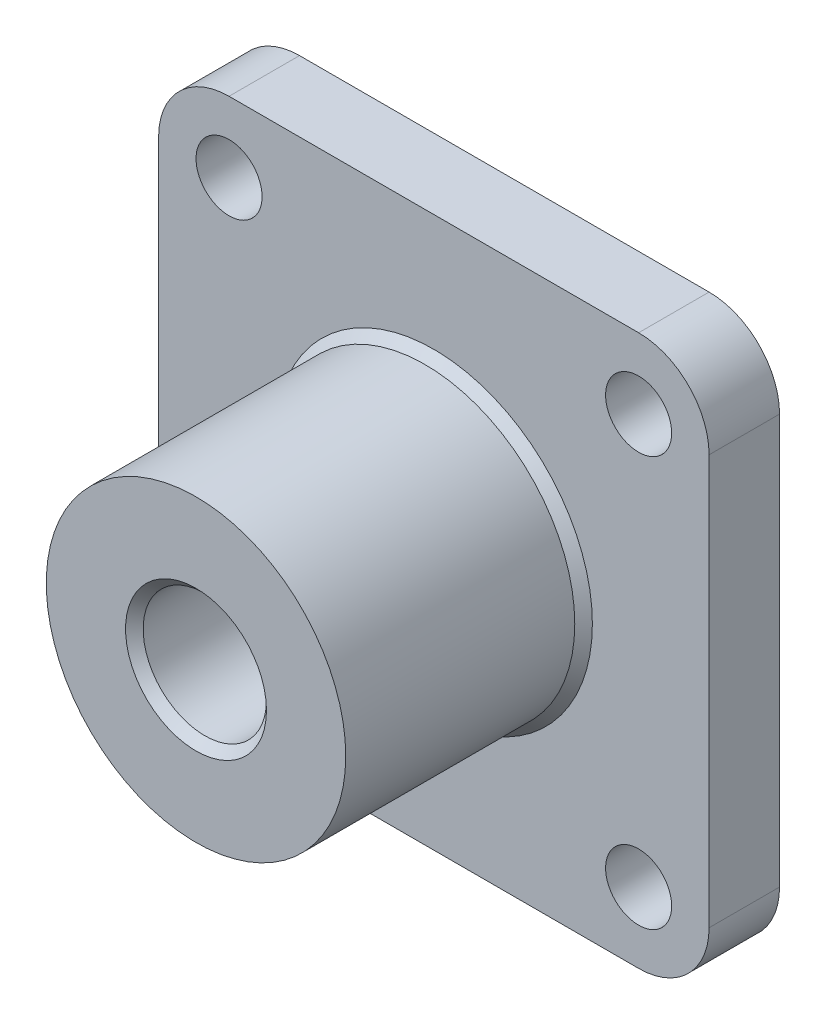
ISO-10303-21;
HEADER;
FILE_DESCRIPTION(('STEP AP214'),'2;1');
FILE_NAME('part.step','',(''),(''),'','','');
FILE_SCHEMA(('AUTOMOTIVE_DESIGN { 1 0 10303 214 1 1 1 1 }'));
ENDSEC;
DATA;
#1=APPLICATION_CONTEXT('core data for automotive mechanical design processes');
#2=APPLICATION_PROTOCOL_DEFINITION('international standard','automotive_design',2000,#1);
#3=PRODUCT_CONTEXT('',#1,'mechanical');
#4=PRODUCT('Part','Part','',(#3));
#5=PRODUCT_RELATED_PRODUCT_CATEGORY('part','',(#4));
#6=PRODUCT_DEFINITION_FORMATION('','',#4);
#7=PRODUCT_DEFINITION_CONTEXT('part definition',#1,'design');
#8=PRODUCT_DEFINITION('design','',#6,#7);
#9=PRODUCT_DEFINITION_SHAPE('','',#8);
#10=(LENGTH_UNIT() NAMED_UNIT(*) SI_UNIT(.MILLI.,.METRE.));
#11=(NAMED_UNIT(*) PLANE_ANGLE_UNIT() SI_UNIT($,.RADIAN.));
#12=(NAMED_UNIT(*) SI_UNIT($,.STERADIAN.) SOLID_ANGLE_UNIT());
#13=UNCERTAINTY_MEASURE_WITH_UNIT(LENGTH_MEASURE(1.E-05),#10,'distance_accuracy_value','');
#14=(GEOMETRIC_REPRESENTATION_CONTEXT(3) GLOBAL_UNCERTAINTY_ASSIGNED_CONTEXT((#13)) GLOBAL_UNIT_ASSIGNED_CONTEXT((#10,
#11,#12)) REPRESENTATION_CONTEXT('',''));
#15=CARTESIAN_POINT('',(0.,0.,0.));
#16=DIRECTION('',(0.,0.,1.));
#17=DIRECTION('',(1.,0.,0.));
#18=AXIS2_PLACEMENT_3D('',#15,#16,#17);
#19=CARTESIAN_POINT('',(16.,-109.,16.));
#20=DIRECTION('',(0.,0.,-1.));
#21=DIRECTION('',(-1.,0.,0.));
#22=AXIS2_PLACEMENT_3D('',#19,#20,#21);
#23=CYLINDRICAL_SURFACE('',#22,16.);
#24=CARTESIAN_POINT('',(16.,-109.,0.));
#25=DIRECTION('',(0.,0.,1.));
#26=DIRECTION('',(1.,0.,0.));
#27=AXIS2_PLACEMENT_3D('',#24,#25,#26);
#28=CIRCLE('',#27,16.);
#29=CARTESIAN_POINT('',(0.,-109.,0.));
#30=VERTEX_POINT('',#29);
#31=CARTESIAN_POINT('',(16.0000000000001,-125.,0.));
#32=VERTEX_POINT('',#31);
#33=EDGE_CURVE('E148',#30,#32,#28,.T.);
#34=ORIENTED_EDGE('',*,*,#33,.T.);
#35=DIRECTION('',(0.,0.,-1.));
#36=VECTOR('',#35,1.);
#37=CARTESIAN_POINT('',(16.0000000000001,-125.,16.));
#38=LINE('',#37,#36);
#39=CARTESIAN_POINT('',(16.0000000000001,-125.,16.));
#40=VERTEX_POINT('',#39);
#41=EDGE_CURVE('E174',#40,#32,#38,.T.);
#42=ORIENTED_EDGE('',*,*,#41,.F.);
#43=CARTESIAN_POINT('',(16.,-109.,16.));
#44=DIRECTION('',(0.,0.,1.));
#45=DIRECTION('',(1.,0.,0.));
#46=AXIS2_PLACEMENT_3D('',#43,#44,#45);
#47=CIRCLE('',#46,16.);
#48=CARTESIAN_POINT('',(0.,-109.,16.));
#49=VERTEX_POINT('',#48);
#50=EDGE_CURVE('E161',#49,#40,#47,.T.);
#51=ORIENTED_EDGE('',*,*,#50,.F.);
#52=DIRECTION('',(0.,0.,-1.));
#53=VECTOR('',#52,1.);
#54=CARTESIAN_POINT('',(0.,-109.,16.));
#55=LINE('',#54,#53);
#56=EDGE_CURVE('E142',#49,#30,#55,.T.);
#57=ORIENTED_EDGE('',*,*,#56,.T.);
#58=EDGE_LOOP('',(#34,#42,#51,#57));
#59=FACE_BOUND('',#58,.T.);
#60=ADVANCED_FACE('F50',(#59),#23,.T.);
#61=CARTESIAN_POINT('',(109.,-125.,16.));
#62=DIRECTION('',(0.,1.,0.));
#63=DIRECTION('',(0.,0.,1.));
#64=AXIS2_PLACEMENT_3D('',#61,#62,#63);
#65=PLANE('',#64);
#66=DIRECTION('',(1.,0.,0.));
#67=VECTOR('',#66,1.);
#68=CARTESIAN_POINT('',(109.,-125.,0.));
#69=LINE('',#68,#67);
#70=CARTESIAN_POINT('',(109.,-125.,0.));
#71=VERTEX_POINT('',#70);
#72=EDGE_CURVE('E149',#32,#71,#69,.T.);
#73=ORIENTED_EDGE('',*,*,#72,.T.);
#74=DIRECTION('',(0.,0.,-1.));
#75=VECTOR('',#74,1.);
#76=CARTESIAN_POINT('',(109.,-125.,16.));
#77=LINE('',#76,#75);
#78=CARTESIAN_POINT('',(109.,-125.,16.));
#79=VERTEX_POINT('',#78);
#80=EDGE_CURVE('E172',#79,#71,#77,.T.);
#81=ORIENTED_EDGE('',*,*,#80,.F.);
#82=DIRECTION('',(1.,0.,0.));
#83=VECTOR('',#82,1.);
#84=CARTESIAN_POINT('',(109.,-125.,16.));
#85=LINE('',#84,#83);
#86=EDGE_CURVE('E108',#40,#79,#85,.T.);
#87=ORIENTED_EDGE('',*,*,#86,.F.);
#88=ORIENTED_EDGE('',*,*,#41,.T.);
#89=EDGE_LOOP('',(#73,#81,#87,#88));
#90=FACE_BOUND('',#89,.T.);
#91=ADVANCED_FACE('F197',(#90),#65,.F.);
#92=CARTESIAN_POINT('',(109.,-109.,16.));
#93=DIRECTION('',(0.,0.,-1.));
#94=DIRECTION('',(-1.,0.,0.));
#95=AXIS2_PLACEMENT_3D('',#92,#93,#94);
#96=CYLINDRICAL_SURFACE('',#95,16.);
#97=CARTESIAN_POINT('',(109.,-109.,0.));
#98=DIRECTION('',(0.,0.,1.));
#99=DIRECTION('',(1.,0.,0.));
#100=AXIS2_PLACEMENT_3D('',#97,#98,#99);
#101=CIRCLE('',#100,16.);
#102=CARTESIAN_POINT('',(125.,-109.,0.));
#103=VERTEX_POINT('',#102);
#104=EDGE_CURVE('E155',#71,#103,#101,.T.);
#105=ORIENTED_EDGE('',*,*,#104,.T.);
#106=DIRECTION('',(0.,0.,-1.));
#107=VECTOR('',#106,1.);
#108=CARTESIAN_POINT('',(125.,-109.,16.));
#109=LINE('',#108,#107);
#110=CARTESIAN_POINT('',(125.,-109.,16.));
#111=VERTEX_POINT('',#110);
#112=EDGE_CURVE('E169',#111,#103,#109,.T.);
#113=ORIENTED_EDGE('',*,*,#112,.F.);
#114=CARTESIAN_POINT('',(109.,-109.,16.));
#115=DIRECTION('',(0.,0.,1.));
#116=DIRECTION('',(1.,0.,0.));
#117=AXIS2_PLACEMENT_3D('',#114,#115,#116);
#118=CIRCLE('',#117,16.);
#119=EDGE_CURVE('E263',#79,#111,#118,.T.);
#120=ORIENTED_EDGE('',*,*,#119,.F.);
#121=ORIENTED_EDGE('',*,*,#80,.T.);
#122=EDGE_LOOP('',(#105,#113,#120,#121));
#123=FACE_BOUND('',#122,.T.);
#124=ADVANCED_FACE('F201',(#123),#96,.T.);
#125=CARTESIAN_POINT('',(125.,-16.0000000000001,16.));
#126=DIRECTION('',(-1.,0.,0.));
#127=DIRECTION('',(0.,0.,1.));
#128=AXIS2_PLACEMENT_3D('',#125,#126,#127);
#129=PLANE('',#128);
#130=DIRECTION('',(0.,1.,0.));
#131=VECTOR('',#130,1.);
#132=CARTESIAN_POINT('',(125.,-16.0000000000001,0.));
#133=LINE('',#132,#131);
#134=CARTESIAN_POINT('',(125.,-16.0000000000001,0.));
#135=VERTEX_POINT('',#134);
#136=EDGE_CURVE('E152',#103,#135,#133,.T.);
#137=ORIENTED_EDGE('',*,*,#136,.T.);
#138=DIRECTION('',(0.,0.,-1.));
#139=VECTOR('',#138,1.);
#140=CARTESIAN_POINT('',(125.,-16.0000000000001,16.));
#141=LINE('',#140,#139);
#142=CARTESIAN_POINT('',(125.,-16.0000000000001,16.));
#143=VERTEX_POINT('',#142);
#144=EDGE_CURVE('E164',#143,#135,#141,.T.);
#145=ORIENTED_EDGE('',*,*,#144,.F.);
#146=DIRECTION('',(0.,1.,0.));
#147=VECTOR('',#146,1.);
#148=CARTESIAN_POINT('',(125.,-16.0000000000001,16.));
#149=LINE('',#148,#147);
#150=EDGE_CURVE('E264',#111,#143,#149,.T.);
#151=ORIENTED_EDGE('',*,*,#150,.F.);
#152=ORIENTED_EDGE('',*,*,#112,.T.);
#153=EDGE_LOOP('',(#137,#145,#151,#152));
#154=FACE_BOUND('',#153,.T.);
#155=ADVANCED_FACE('F271',(#154),#129,.F.);
#156=CARTESIAN_POINT('',(109.,-16.,16.));
#157=DIRECTION('',(0.,0.,-1.));
#158=DIRECTION('',(-1.,0.,0.));
#159=AXIS2_PLACEMENT_3D('',#156,#157,#158);
#160=CYLINDRICAL_SURFACE('',#159,16.);
#161=CARTESIAN_POINT('',(109.,-16.,0.));
#162=DIRECTION('',(0.,0.,1.));
#163=DIRECTION('',(1.,0.,0.));
#164=AXIS2_PLACEMENT_3D('',#161,#162,#163);
#165=CIRCLE('',#164,16.);
#166=CARTESIAN_POINT('',(109.,0.,0.));
#167=VERTEX_POINT('',#166);
#168=EDGE_CURVE('E156',#135,#167,#165,.T.);
#169=ORIENTED_EDGE('',*,*,#168,.T.);
#170=DIRECTION('',(0.,0.,-1.));
#171=VECTOR('',#170,1.);
#172=CARTESIAN_POINT('',(109.,0.,16.));
#173=LINE('',#172,#171);
#174=CARTESIAN_POINT('',(109.,0.,16.));
#175=VERTEX_POINT('',#174);
#176=EDGE_CURVE('E136',#175,#167,#173,.T.);
#177=ORIENTED_EDGE('',*,*,#176,.F.);
#178=CARTESIAN_POINT('',(109.,-16.,16.));
#179=DIRECTION('',(0.,0.,1.));
#180=DIRECTION('',(1.,0.,0.));
#181=AXIS2_PLACEMENT_3D('',#178,#179,#180);
#182=CIRCLE('',#181,16.);
#183=EDGE_CURVE('E126',#143,#175,#182,.T.);
#184=ORIENTED_EDGE('',*,*,#183,.F.);
#185=ORIENTED_EDGE('',*,*,#144,.T.);
#186=EDGE_LOOP('',(#169,#177,#184,#185));
#187=FACE_BOUND('',#186,.T.);
#188=ADVANCED_FACE('F274',(#187),#160,.T.);
#189=CARTESIAN_POINT('',(16.0000000000001,0.,16.));
#190=DIRECTION('',(0.,-1.,0.));
#191=DIRECTION('',(0.,0.,-1.));
#192=AXIS2_PLACEMENT_3D('',#189,#190,#191);
#193=PLANE('',#192);
#194=DIRECTION('',(-1.,0.,0.));
#195=VECTOR('',#194,1.);
#196=CARTESIAN_POINT('',(16.0000000000001,0.,0.));
#197=LINE('',#196,#195);
#198=CARTESIAN_POINT('',(16.0000000000001,0.,0.));
#199=VERTEX_POINT('',#198);
#200=EDGE_CURVE('E139',#167,#199,#197,.T.);
#201=ORIENTED_EDGE('',*,*,#200,.T.);
#202=DIRECTION('',(0.,0.,-1.));
#203=VECTOR('',#202,1.);
#204=CARTESIAN_POINT('',(16.0000000000001,0.,16.));
#205=LINE('',#204,#203);
#206=CARTESIAN_POINT('',(16.0000000000001,0.,16.));
#207=VERTEX_POINT('',#206);
#208=EDGE_CURVE('E133',#207,#199,#205,.T.);
#209=ORIENTED_EDGE('',*,*,#208,.F.);
#210=DIRECTION('',(-1.,0.,0.));
#211=VECTOR('',#210,1.);
#212=CARTESIAN_POINT('',(16.0000000000001,0.,16.));
#213=LINE('',#212,#211);
#214=EDGE_CURVE('E121',#175,#207,#213,.T.);
#215=ORIENTED_EDGE('',*,*,#214,.F.);
#216=ORIENTED_EDGE('',*,*,#176,.T.);
#217=EDGE_LOOP('',(#201,#209,#215,#216));
#218=FACE_BOUND('',#217,.T.);
#219=ADVANCED_FACE('F134',(#218),#193,.F.);
#220=CARTESIAN_POINT('',(16.,-16.,16.));
#221=DIRECTION('',(0.,0.,-1.));
#222=DIRECTION('',(-1.,0.,0.));
#223=AXIS2_PLACEMENT_3D('',#220,#221,#222);
#224=CYLINDRICAL_SURFACE('',#223,16.);
#225=CARTESIAN_POINT('',(16.,-16.,0.));
#226=DIRECTION('',(0.,0.,1.));
#227=DIRECTION('',(-1.,0.,0.));
#228=AXIS2_PLACEMENT_3D('',#225,#226,#227);
#229=CIRCLE('',#228,16.);
#230=CARTESIAN_POINT('',(0.,-16.0000000000001,0.));
#231=VERTEX_POINT('',#230);
#232=EDGE_CURVE('E94',#199,#231,#229,.T.);
#233=ORIENTED_EDGE('',*,*,#232,.T.);
#234=DIRECTION('',(0.,0.,-1.));
#235=VECTOR('',#234,1.);
#236=CARTESIAN_POINT('',(0.,-16.0000000000001,16.));
#237=LINE('',#236,#235);
#238=CARTESIAN_POINT('',(0.,-16.0000000000001,16.));
#239=VERTEX_POINT('',#238);
#240=EDGE_CURVE('E140',#239,#231,#237,.T.);
#241=ORIENTED_EDGE('',*,*,#240,.F.);
#242=CARTESIAN_POINT('',(16.,-16.,16.));
#243=DIRECTION('',(0.,0.,1.));
#244=DIRECTION('',(-1.,0.,0.));
#245=AXIS2_PLACEMENT_3D('',#242,#243,#244);
#246=CIRCLE('',#245,16.);
#247=EDGE_CURVE('E127',#207,#239,#246,.T.);
#248=ORIENTED_EDGE('',*,*,#247,.F.);
#249=ORIENTED_EDGE('',*,*,#208,.T.);
#250=EDGE_LOOP('',(#233,#241,#248,#249));
#251=FACE_BOUND('',#250,.T.);
#252=ADVANCED_FACE('F137',(#251),#224,.T.);
#253=CARTESIAN_POINT('',(0.,-109.,16.));
#254=DIRECTION('',(1.,0.,0.));
#255=DIRECTION('',(0.,0.,-1.));
#256=AXIS2_PLACEMENT_3D('',#253,#254,#255);
#257=PLANE('',#256);
#258=DIRECTION('',(0.,-1.,0.));
#259=VECTOR('',#258,1.);
#260=CARTESIAN_POINT('',(0.,-109.,0.));
#261=LINE('',#260,#259);
#262=EDGE_CURVE('E99',#231,#30,#261,.T.);
#263=ORIENTED_EDGE('',*,*,#262,.T.);
#264=ORIENTED_EDGE('',*,*,#56,.F.);
#265=DIRECTION('',(0.,-1.,0.));
#266=VECTOR('',#265,1.);
#267=CARTESIAN_POINT('',(0.,-109.,16.));
#268=LINE('',#267,#266);
#269=EDGE_CURVE('E61',#239,#49,#268,.T.);
#270=ORIENTED_EDGE('',*,*,#269,.F.);
#271=ORIENTED_EDGE('',*,*,#240,.T.);
#272=EDGE_LOOP('',(#263,#264,#270,#271));
#273=FACE_BOUND('',#272,.T.);
#274=ADVANCED_FACE('F285',(#273),#257,.F.);
#275=CARTESIAN_POINT('',(16.,-109.,16.));
#276=DIRECTION('',(0.,0.,1.));
#277=DIRECTION('',(1.,0.,0.));
#278=AXIS2_PLACEMENT_3D('',#275,#276,#277);
#279=PLANE('',#278);
#280=CARTESIAN_POINT('',(62.5,-62.5,16.));
#281=DIRECTION('',(0.,0.,1.));
#282=DIRECTION('',(1.,0.,0.));
#283=AXIS2_PLACEMENT_3D('',#280,#281,#282);
#284=CIRCLE('',#283,36.);
#285=CARTESIAN_POINT('',(98.5,-62.5,16.));
#286=VERTEX_POINT('',#285);
#287=EDGE_CURVE('E178',#286,#286,#284,.F.);
#288=ORIENTED_EDGE('',*,*,#287,.T.);
#289=EDGE_LOOP('',(#288));
#290=FACE_BOUND('',#289,.T.);
#291=CARTESIAN_POINT('',(16.,-109.,16.));
#292=DIRECTION('',(0.,0.,1.));
#293=DIRECTION('',(1.,0.,0.));
#294=AXIS2_PLACEMENT_3D('',#291,#292,#293);
#295=CIRCLE('',#294,7.50000000000001);
#296=CARTESIAN_POINT('',(23.5,-109.,16.));
#297=VERTEX_POINT('',#296);
#298=EDGE_CURVE('E235',#297,#297,#295,.T.);
#299=ORIENTED_EDGE('',*,*,#298,.F.);
#300=EDGE_LOOP('',(#299));
#301=FACE_BOUND('',#300,.T.);
#302=CARTESIAN_POINT('',(109.,-109.,16.));
#303=DIRECTION('',(0.,0.,1.));
#304=DIRECTION('',(1.,0.,0.));
#305=AXIS2_PLACEMENT_3D('',#302,#303,#304);
#306=CIRCLE('',#305,7.5);
#307=CARTESIAN_POINT('',(116.5,-109.,16.));
#308=VERTEX_POINT('',#307);
#309=EDGE_CURVE('E252',#308,#308,#306,.T.);
#310=ORIENTED_EDGE('',*,*,#309,.F.);
#311=EDGE_LOOP('',(#310));
#312=FACE_BOUND('',#311,.T.);
#313=CARTESIAN_POINT('',(109.,-16.,16.));
#314=DIRECTION('',(0.,0.,1.));
#315=DIRECTION('',(1.,0.,0.));
#316=AXIS2_PLACEMENT_3D('',#313,#314,#315);
#317=CIRCLE('',#316,7.5);
#318=CARTESIAN_POINT('',(116.5,-16.,16.));
#319=VERTEX_POINT('',#318);
#320=EDGE_CURVE('E249',#319,#319,#317,.T.);
#321=ORIENTED_EDGE('',*,*,#320,.F.);
#322=EDGE_LOOP('',(#321));
#323=FACE_BOUND('',#322,.T.);
#324=CARTESIAN_POINT('',(16.,-16.,16.));
#325=DIRECTION('',(0.,0.,1.));
#326=DIRECTION('',(1.,0.,0.));
#327=AXIS2_PLACEMENT_3D('',#324,#325,#326);
#328=CIRCLE('',#327,7.5);
#329=CARTESIAN_POINT('',(23.5,-16.,16.));
#330=VERTEX_POINT('',#329);
#331=EDGE_CURVE('E241',#330,#330,#328,.T.);
#332=ORIENTED_EDGE('',*,*,#331,.F.);
#333=EDGE_LOOP('',(#332));
#334=FACE_BOUND('',#333,.T.);
#335=ORIENTED_EDGE('',*,*,#50,.T.);
#336=ORIENTED_EDGE('',*,*,#86,.T.);
#337=ORIENTED_EDGE('',*,*,#119,.T.);
#338=ORIENTED_EDGE('',*,*,#150,.T.);
#339=ORIENTED_EDGE('',*,*,#183,.T.);
#340=ORIENTED_EDGE('',*,*,#214,.T.);
#341=ORIENTED_EDGE('',*,*,#247,.T.);
#342=ORIENTED_EDGE('',*,*,#269,.T.);
#343=EDGE_LOOP('',(#335,#336,#337,#338,#339,#340,#341,#342));
#344=FACE_BOUND('',#343,.T.);
#345=ADVANCED_FACE('F123',(#290,#301,#312,#323,#334,#344),#279,.T.);
#346=CARTESIAN_POINT('',(16.,-109.,0.));
#347=DIRECTION('',(0.,0.,1.));
#348=DIRECTION('',(1.,0.,0.));
#349=AXIS2_PLACEMENT_3D('',#346,#347,#348);
#350=PLANE('',#349);
#351=CARTESIAN_POINT('',(16.,-109.,0.));
#352=DIRECTION('',(0.,0.,1.));
#353=DIRECTION('',(1.,0.,0.));
#354=AXIS2_PLACEMENT_3D('',#351,#352,#353);
#355=CIRCLE('',#354,7.50000000000001);
#356=CARTESIAN_POINT('',(23.5,-109.,0.));
#357=VERTEX_POINT('',#356);
#358=EDGE_CURVE('E240',#357,#357,#355,.T.);
#359=ORIENTED_EDGE('',*,*,#358,.T.);
#360=EDGE_LOOP('',(#359));
#361=FACE_BOUND('',#360,.T.);
#362=CARTESIAN_POINT('',(109.,-109.,0.));
#363=DIRECTION('',(0.,0.,1.));
#364=DIRECTION('',(1.,0.,0.));
#365=AXIS2_PLACEMENT_3D('',#362,#363,#364);
#366=CIRCLE('',#365,7.5);
#367=CARTESIAN_POINT('',(116.5,-109.,0.));
#368=VERTEX_POINT('',#367);
#369=EDGE_CURVE('E248',#368,#368,#366,.T.);
#370=ORIENTED_EDGE('',*,*,#369,.T.);
#371=EDGE_LOOP('',(#370));
#372=FACE_BOUND('',#371,.T.);
#373=CARTESIAN_POINT('',(109.,-16.,0.));
#374=DIRECTION('',(0.,0.,1.));
#375=DIRECTION('',(1.,0.,0.));
#376=AXIS2_PLACEMENT_3D('',#373,#374,#375);
#377=CIRCLE('',#376,7.5);
#378=CARTESIAN_POINT('',(116.5,-16.,0.));
#379=VERTEX_POINT('',#378);
#380=EDGE_CURVE('E245',#379,#379,#377,.T.);
#381=ORIENTED_EDGE('',*,*,#380,.T.);
#382=EDGE_LOOP('',(#381));
#383=FACE_BOUND('',#382,.T.);
#384=CARTESIAN_POINT('',(16.,-16.,0.));
#385=DIRECTION('',(0.,0.,1.));
#386=DIRECTION('',(1.,0.,0.));
#387=AXIS2_PLACEMENT_3D('',#384,#385,#386);
#388=CIRCLE('',#387,7.5);
#389=CARTESIAN_POINT('',(23.5,-16.,0.));
#390=VERTEX_POINT('',#389);
#391=EDGE_CURVE('E147',#390,#390,#388,.T.);
#392=ORIENTED_EDGE('',*,*,#391,.T.);
#393=EDGE_LOOP('',(#392));
#394=FACE_BOUND('',#393,.T.);
#395=ORIENTED_EDGE('',*,*,#33,.F.);
#396=ORIENTED_EDGE('',*,*,#262,.F.);
#397=ORIENTED_EDGE('',*,*,#232,.F.);
#398=ORIENTED_EDGE('',*,*,#200,.F.);
#399=ORIENTED_EDGE('',*,*,#168,.F.);
#400=ORIENTED_EDGE('',*,*,#136,.F.);
#401=ORIENTED_EDGE('',*,*,#104,.F.);
#402=ORIENTED_EDGE('',*,*,#72,.F.);
#403=EDGE_LOOP('',(#395,#396,#397,#398,#399,#400,#401,#402));
#404=FACE_BOUND('',#403,.T.);
#405=ADVANCED_FACE('F279',(#361,#372,#383,#394,#404),#350,.F.);
#406=CARTESIAN_POINT('',(16.,-16.,0.));
#407=DIRECTION('',(0.,0.,1.));
#408=DIRECTION('',(1.,0.,0.));
#409=AXIS2_PLACEMENT_3D('',#406,#407,#408);
#410=CYLINDRICAL_SURFACE('',#409,7.5);
#411=ORIENTED_EDGE('',*,*,#391,.F.);
#412=EDGE_LOOP('',(#411));
#413=FACE_BOUND('',#412,.T.);
#414=ORIENTED_EDGE('',*,*,#331,.T.);
#415=EDGE_LOOP('',(#414));
#416=FACE_BOUND('',#415,.T.);
#417=ADVANCED_FACE('F334',(#413,#416),#410,.F.);
#418=CARTESIAN_POINT('',(109.,-16.,0.));
#419=DIRECTION('',(0.,0.,1.));
#420=DIRECTION('',(1.,0.,0.));
#421=AXIS2_PLACEMENT_3D('',#418,#419,#420);
#422=CYLINDRICAL_SURFACE('',#421,7.5);
#423=ORIENTED_EDGE('',*,*,#380,.F.);
#424=EDGE_LOOP('',(#423));
#425=FACE_BOUND('',#424,.T.);
#426=ORIENTED_EDGE('',*,*,#320,.T.);
#427=EDGE_LOOP('',(#426));
#428=FACE_BOUND('',#427,.T.);
#429=ADVANCED_FACE('F340',(#425,#428),#422,.F.);
#430=CARTESIAN_POINT('',(109.,-109.,0.));
#431=DIRECTION('',(0.,0.,1.));
#432=DIRECTION('',(1.,0.,0.));
#433=AXIS2_PLACEMENT_3D('',#430,#431,#432);
#434=CYLINDRICAL_SURFACE('',#433,7.5);
#435=ORIENTED_EDGE('',*,*,#369,.F.);
#436=EDGE_LOOP('',(#435));
#437=FACE_BOUND('',#436,.T.);
#438=ORIENTED_EDGE('',*,*,#309,.T.);
#439=EDGE_LOOP('',(#438));
#440=FACE_BOUND('',#439,.T.);
#441=ADVANCED_FACE('F346',(#437,#440),#434,.F.);
#442=CARTESIAN_POINT('',(16.,-109.,0.));
#443=DIRECTION('',(0.,0.,1.));
#444=DIRECTION('',(1.,0.,0.));
#445=AXIS2_PLACEMENT_3D('',#442,#443,#444);
#446=CYLINDRICAL_SURFACE('',#445,7.50000000000001);
#447=ORIENTED_EDGE('',*,*,#358,.F.);
#448=EDGE_LOOP('',(#447));
#449=FACE_BOUND('',#448,.T.);
#450=ORIENTED_EDGE('',*,*,#298,.T.);
#451=EDGE_LOOP('',(#450));
#452=FACE_BOUND('',#451,.T.);
#453=ADVANCED_FACE('F230',(#449,#452),#446,.F.);
#454=CARTESIAN_POINT('',(62.5,-62.5,70.));
#455=DIRECTION('',(0.,0.,-1.));
#456=DIRECTION('',(-1.,0.,0.));
#457=AXIS2_PLACEMENT_3D('',#454,#455,#456);
#458=CYLINDRICAL_SURFACE('',#457,34.);
#459=CARTESIAN_POINT('',(62.5,-62.5,18.));
#460=DIRECTION('',(0.,0.,1.));
#461=DIRECTION('',(1.,0.,0.));
#462=AXIS2_PLACEMENT_3D('',#459,#460,#461);
#463=CIRCLE('',#462,34.);
#464=CARTESIAN_POINT('',(96.5,-62.5,18.));
#465=VERTEX_POINT('',#464);
#466=EDGE_CURVE('E179',#465,#465,#463,.T.);
#467=ORIENTED_EDGE('',*,*,#466,.T.);
#468=EDGE_LOOP('',(#467));
#469=FACE_BOUND('',#468,.T.);
#470=CARTESIAN_POINT('',(62.5,-62.5,70.));
#471=DIRECTION('',(0.,0.,1.));
#472=DIRECTION('',(1.,0.,0.));
#473=AXIS2_PLACEMENT_3D('',#470,#471,#472);
#474=CIRCLE('',#473,34.);
#475=CARTESIAN_POINT('',(96.5,-62.5,70.));
#476=VERTEX_POINT('',#475);
#477=EDGE_CURVE('E234',#476,#476,#474,.T.);
#478=ORIENTED_EDGE('',*,*,#477,.F.);
#479=EDGE_LOOP('',(#478));
#480=FACE_BOUND('',#479,.T.);
#481=ADVANCED_FACE('F218',(#469,#480),#458,.T.);
#482=CARTESIAN_POINT('',(62.5,-62.5,70.));
#483=DIRECTION('',(0.,0.,1.));
#484=DIRECTION('',(1.,0.,0.));
#485=AXIS2_PLACEMENT_3D('',#482,#483,#484);
#486=PLANE('',#485);
#487=CARTESIAN_POINT('',(62.5,-62.5,70.));
#488=DIRECTION('',(0.,0.,1.));
#489=DIRECTION('',(1.,0.,0.));
#490=AXIS2_PLACEMENT_3D('',#487,#488,#489);
#491=CIRCLE('',#490,16.);
#492=CARTESIAN_POINT('',(78.5,-62.5,70.));
#493=VERTEX_POINT('',#492);
#494=EDGE_CURVE('E11',#493,#493,#491,.F.);
#495=ORIENTED_EDGE('',*,*,#494,.T.);
#496=EDGE_LOOP('',(#495));
#497=FACE_BOUND('',#496,.T.);
#498=ORIENTED_EDGE('',*,*,#477,.T.);
#499=EDGE_LOOP('',(#498));
#500=FACE_BOUND('',#499,.T.);
#501=ADVANCED_FACE('F211',(#497,#500),#486,.T.);
#502=CARTESIAN_POINT('',(62.5,-62.5,18.));
#503=DIRECTION('',(0.,0.,-1.));
#504=DIRECTION('',(-1.,0.,0.));
#505=AXIS2_PLACEMENT_3D('',#502,#503,#504);
#506=CONICAL_SURFACE('',#505,34.,0.785398163397445);
#507=ORIENTED_EDGE('',*,*,#287,.F.);
#508=EDGE_LOOP('',(#507));
#509=FACE_BOUND('',#508,.T.);
#510=ORIENTED_EDGE('',*,*,#466,.F.);
#511=EDGE_LOOP('',(#510));
#512=FACE_BOUND('',#511,.T.);
#513=ADVANCED_FACE('F210',(#509,#512),#506,.T.);
#514=CARTESIAN_POINT('',(62.5,-62.5,16.));
#515=DIRECTION('',(0.,0.,1.));
#516=DIRECTION('',(1.,0.,0.));
#517=AXIS2_PLACEMENT_3D('',#514,#515,#516);
#518=CYLINDRICAL_SURFACE('',#517,14.);
#519=CARTESIAN_POINT('',(62.5,-62.5,68.));
#520=DIRECTION('',(0.,0.,1.));
#521=DIRECTION('',(1.,0.,0.));
#522=AXIS2_PLACEMENT_3D('',#519,#520,#521);
#523=CIRCLE('',#522,14.);
#524=CARTESIAN_POINT('',(76.5,-62.5,68.));
#525=VERTEX_POINT('',#524);
#526=EDGE_CURVE('E60',#525,#525,#523,.T.);
#527=ORIENTED_EDGE('',*,*,#526,.T.);
#528=EDGE_LOOP('',(#527));
#529=FACE_BOUND('',#528,.T.);
#530=CARTESIAN_POINT('',(62.5,-62.5,16.));
#531=DIRECTION('',(0.,0.,1.));
#532=DIRECTION('',(1.,0.,0.));
#533=AXIS2_PLACEMENT_3D('',#530,#531,#532);
#534=CIRCLE('',#533,14.);
#535=CARTESIAN_POINT('',(76.5,-62.5,16.));
#536=VERTEX_POINT('',#535);
#537=EDGE_CURVE('E233',#536,#536,#534,.T.);
#538=ORIENTED_EDGE('',*,*,#537,.F.);
#539=EDGE_LOOP('',(#538));
#540=FACE_BOUND('',#539,.T.);
#541=ADVANCED_FACE('F184',(#529,#540),#518,.F.);
#542=CARTESIAN_POINT('',(62.5,-62.5,16.));
#543=DIRECTION('',(0.,0.,1.));
#544=DIRECTION('',(1.,0.,0.));
#545=AXIS2_PLACEMENT_3D('',#542,#543,#544);
#546=PLANE('',#545);
#547=ORIENTED_EDGE('',*,*,#537,.T.);
#548=EDGE_LOOP('',(#547));
#549=FACE_BOUND('',#548,.T.);
#550=ADVANCED_FACE('F188',(#549),#546,.T.);
#551=CARTESIAN_POINT('',(62.5,-62.5,68.));
#552=DIRECTION('',(0.,0.,1.));
#553=DIRECTION('',(1.,0.,0.));
#554=AXIS2_PLACEMENT_3D('',#551,#552,#553);
#555=CONICAL_SURFACE('',#554,14.,0.785398163397452);
#556=ORIENTED_EDGE('',*,*,#494,.F.);
#557=EDGE_LOOP('',(#556));
#558=FACE_BOUND('',#557,.T.);
#559=ORIENTED_EDGE('',*,*,#526,.F.);
#560=EDGE_LOOP('',(#559));
#561=FACE_BOUND('',#560,.T.);
#562=ADVANCED_FACE('F49',(#558,#561),#555,.F.);
#563=CLOSED_SHELL('',(#60,#91,#124,#155,#188,#219,#252,#274,#345,#405,#417,#429,#441,#453,#481,
#501,#513,#541,#550,#562));
#564=MANIFOLD_SOLID_BREP('B2',#563);
#565=ADVANCED_BREP_SHAPE_REPRESENTATION('',(#18,#564),#14);
#566=SHAPE_DEFINITION_REPRESENTATION(#9,#565);
ENDSEC;
END-ISO-10303-21;
